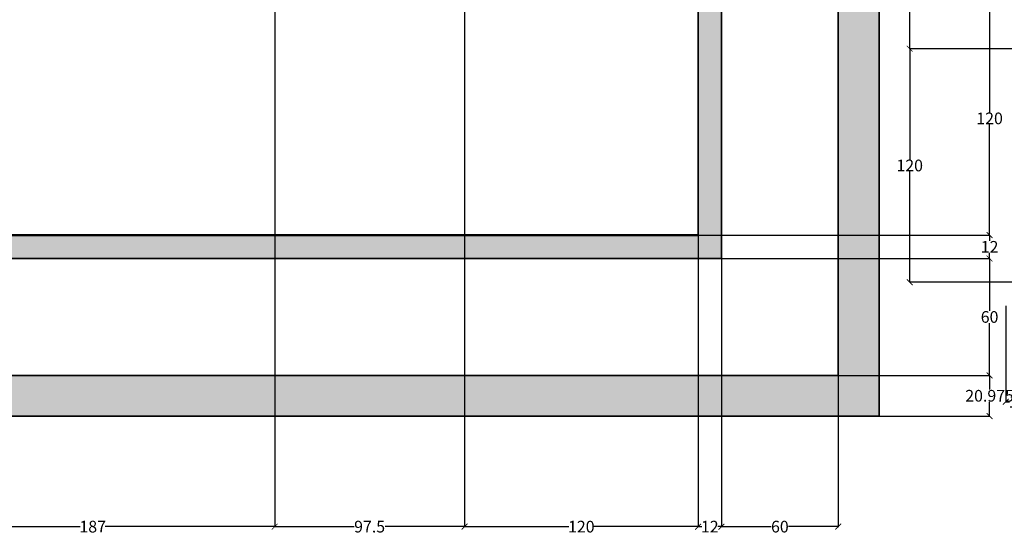
# Model space of a CAD drawing. Units: inches. Extents: x 925 to 2834, y 111 to 1355.
# Tile 5 of 25: x 1490 to 1996, y 111 to 376. Entities that reach past the tile are written whole.
import ezdxf

# ---------------------------------------------------------------- set-up
doc = ezdxf.new("R2010")
doc.units = ezdxf.units.IN
doc.header["$MEASUREMENT"] = 0
for name, color, linetype, lineweight in [('A-ANNO-DIMS', 2, 'Continuous', 18), ('A-ANNO-TTLB', 7, 'Continuous', 35), ('A-FLOR-PATT', 252, 'Continuous', 13), ('A-WALL', 7, 'Continuous', 50)]:
    doc.layers.add(name, color=color, linetype=linetype, lineweight=lineweight)
doc.styles.get("Standard").update_dxf_attribs({"font": 'arial.ttf'})
doc.dimstyles.get("Standard").update_dxf_attribs({"dimtxt": 6, "dimasz": 3, "dimexe": 0.18, "dimexo": 0.0625, "dimgap": 0.09, "dimtad": 0, "dimtih": 1, "dimtoh": 1, "dimdec": 1, "dimzin": 0, "dimdsep": 46, "dimlunit": 3, "dimtxsty": 'Standard', "dimblk": 'ARCHTICK', "dimcen": 0.09, "dimadec": 0, "dimazin": 0, "dimtfac": 1, "dimtdec": 1, "dimtofl": 0, "dimtmove": 0, "dimatfit": 3, "dimfxl": 1, "dimtolj": 1, "dimtzin": 0, "dimarcsym": 0})

# ---------------------------------------------------------------- blocks, each defined once
blk = doc.blocks.new('_ArchTick')
at = {"color": 0, "linetype": 'ByBlock', "const_width": 0.15}
blk.add_lwpolyline([(-0.5, -0.5), (0.5, 0.5)], dxfattribs=at)
blk = doc.blocks.new('*D27')
at = {"layer": 'A-ANNO-DIMS', "color": 0, "lineweight": -2, "transparency": 16777216}
for p, q in [((1621.21, 395.03), (1621.21, 115.18)), ((1434.21, 385.03), (1434.21, 115.18)), ((1434.21, 115.36), (1521.28, 115.36)), ((1621.21, 115.36), (1534.15, 115.36))]:
    blk.add_line(p, q, dxfattribs=at)
at = {"layer": 'Defpoints', "color": 0, "transparency": 16777216}
for p in [(1621.21, 395.09), (1434.21, 385.09), (1621.21, 115.36)]:
    blk.add_point(p, dxfattribs=at)
at = {"layer": 'A-ANNO-DIMS', "color": 0, "lineweight": -2, "transparency": 16777216, "xscale": 3, "yscale": 3, "zscale": 3, "rotation": 180}
blk.add_blockref('_ArchTick', (1434.21, 115.36), dxfattribs=at)
at = {"layer": 'A-ANNO-DIMS', "color": 0, "lineweight": -2, "transparency": 16777216, "xscale": 3, "yscale": 3, "zscale": 3}
blk.add_blockref('_ArchTick', (1621.21, 115.36), dxfattribs=at)
at = {"layer": 'A-ANNO-DIMS', "color": 0, "transparency": 16777216, "insert": (1527.71, 115.36), "char_height": 6, "attachment_point": 5}
blk.add_mtext('\\A1;187', dxfattribs=at)
blk = doc.blocks.new('*D28')
at = {"layer": 'A-ANNO-DIMS', "color": 0, "lineweight": -2, "transparency": 16777216}
for p, q in [((1621.21, 395.03), (1621.21, 115.18)), ((1718.71, 385.03), (1718.71, 115.18)), ((1621.21, 115.36), (1662.06, 115.36)), ((1718.71, 115.36), (1677.87, 115.36))]:
    blk.add_line(p, q, dxfattribs=at)
at = {"layer": 'Defpoints', "color": 0, "transparency": 16777216}
for p in [(1621.21, 395.09), (1718.71, 385.09), (1718.71, 115.36)]:
    blk.add_point(p, dxfattribs=at)
at = {"layer": 'A-ANNO-DIMS', "color": 0, "lineweight": -2, "transparency": 16777216, "xscale": 3, "yscale": 3, "zscale": 3, "rotation": 180}
blk.add_blockref('_ArchTick', (1621.21, 115.36), dxfattribs=at)
at = {"layer": 'A-ANNO-DIMS', "color": 0, "lineweight": -2, "transparency": 16777216, "xscale": 3, "yscale": 3, "zscale": 3}
blk.add_blockref('_ArchTick', (1718.71, 115.36), dxfattribs=at)
at = {"layer": 'A-ANNO-DIMS', "color": 0, "transparency": 16777216, "insert": (1669.96, 115.36), "char_height": 6, "attachment_point": 5}
blk.add_mtext('\\A1;97.5', dxfattribs=at)
blk = doc.blocks.new('*D29')
at = {"layer": 'A-ANNO-DIMS', "color": 0, "lineweight": -2, "transparency": 16777216}
for p, q in [((1718.71, 385.03), (1718.71, 115.18)), ((1838.71, 265.03), (1838.71, 115.18)), ((1718.71, 115.36), (1772.29, 115.36)), ((1838.71, 115.36), (1785.14, 115.36))]:
    blk.add_line(p, q, dxfattribs=at)
at = {"layer": 'Defpoints', "color": 0, "transparency": 16777216}
for p in [(1718.71, 385.09), (1838.71, 265.09), (1838.71, 115.36)]:
    blk.add_point(p, dxfattribs=at)
at = {"layer": 'A-ANNO-DIMS', "color": 0, "lineweight": -2, "transparency": 16777216, "xscale": 3, "yscale": 3, "zscale": 3, "rotation": 180}
blk.add_blockref('_ArchTick', (1718.71, 115.36), dxfattribs=at)
at = {"layer": 'A-ANNO-DIMS', "color": 0, "lineweight": -2, "transparency": 16777216, "xscale": 3, "yscale": 3, "zscale": 3}
blk.add_blockref('_ArchTick', (1838.71, 115.36), dxfattribs=at)
at = {"layer": 'A-ANNO-DIMS', "color": 0, "transparency": 16777216, "insert": (1778.71, 115.36), "char_height": 6, "attachment_point": 5}
blk.add_mtext('\\A1;120', dxfattribs=at)
blk = doc.blocks.new('*D30')
at = {"layer": 'A-ANNO-DIMS', "color": 0, "lineweight": -2, "transparency": 16777216}
for p, q in [((1838.71, 265.03), (1838.71, 115.18)), ((1850.71, 253.03), (1850.71, 115.18)), ((1838.71, 115.36), (1840.64, 115.36)), ((1850.71, 115.36), (1848.79, 115.36))]:
    blk.add_line(p, q, dxfattribs=at)
at = {"layer": 'Defpoints', "color": 0, "transparency": 16777216}
for p in [(1838.71, 265.09), (1850.71, 253.09), (1850.71, 115.36)]:
    blk.add_point(p, dxfattribs=at)
at = {"layer": 'A-ANNO-DIMS', "color": 0, "lineweight": -2, "transparency": 16777216, "xscale": 3, "yscale": 3, "zscale": 3, "rotation": 180}
blk.add_blockref('_ArchTick', (1838.71, 115.36), dxfattribs=at)
at = {"layer": 'A-ANNO-DIMS', "color": 0, "lineweight": -2, "transparency": 16777216, "xscale": 3, "yscale": 3, "zscale": 3}
blk.add_blockref('_ArchTick', (1850.71, 115.36), dxfattribs=at)
at = {"layer": 'A-ANNO-DIMS', "color": 0, "transparency": 16777216, "insert": (1844.71, 115.36), "char_height": 6, "attachment_point": 5}
blk.add_mtext('\\A1;12', dxfattribs=at)
blk = doc.blocks.new('*D31')
at = {"layer": 'A-ANNO-DIMS', "color": 0, "lineweight": -2, "transparency": 16777216}
for p, q in [((1850.71, 253.03), (1850.71, 115.18)), ((1910.71, 193.03), (1910.71, 115.18)), ((1850.71, 115.36), (1876.32, 115.36)), ((1910.71, 115.36), (1885.11, 115.36))]:
    blk.add_line(p, q, dxfattribs=at)
at = {"layer": 'Defpoints', "color": 0, "transparency": 16777216}
for p in [(1850.71, 253.09), (1910.71, 193.09), (1910.71, 115.36)]:
    blk.add_point(p, dxfattribs=at)
at = {"layer": 'A-ANNO-DIMS', "color": 0, "lineweight": -2, "transparency": 16777216, "xscale": 3, "yscale": 3, "zscale": 3, "rotation": 180}
blk.add_blockref('_ArchTick', (1850.71, 115.36), dxfattribs=at)
at = {"layer": 'A-ANNO-DIMS', "color": 0, "lineweight": -2, "transparency": 16777216, "xscale": 3, "yscale": 3, "zscale": 3}
blk.add_blockref('_ArchTick', (1910.71, 115.36), dxfattribs=at)
at = {"layer": 'A-ANNO-DIMS', "color": 0, "transparency": 16777216, "insert": (1880.71, 115.36), "char_height": 6, "attachment_point": 5}
blk.add_mtext('\\A1;60', dxfattribs=at)
blk = doc.blocks.new('*D40')
at = {"layer": 'A-ANNO-DIMS', "color": 0, "lineweight": -2, "transparency": 16777216}
for p, q in [((1910.78, 193.09), (1988.62, 193.09)), ((1988.44, 193.09), (1988.44, 185.75)), ((1988.44, 172.11), (1988.44, 179.45)), ((1931.75, 172.11), (1988.62, 172.11))]:
    blk.add_line(p, q, dxfattribs=at)
at = {"layer": 'Defpoints', "color": 0, "transparency": 16777216}
for p in [(1910.71, 193.09), (1988.44, 193.09), (1931.69, 172.11)]:
    blk.add_point(p, dxfattribs=at)
at = {"layer": 'A-ANNO-DIMS', "color": 0, "lineweight": -2, "transparency": 16777216, "xscale": 3, "yscale": 3, "zscale": 3}
for p, rotation in [((1988.44, 193.09), 90), ((1988.44, 172.11), 270)]:
    blk.add_blockref('_ArchTick', p, dxfattribs=dict(at, rotation=rotation))
at = {"layer": 'A-ANNO-DIMS', "color": 0, "transparency": 16777216, "insert": (1988.44, 182.6), "char_height": 6, "attachment_point": 5}
blk.add_mtext('\\A1;20.975', dxfattribs=at)
blk = doc.blocks.new('*D41')
at = {"layer": 'A-ANNO-DIMS', "color": 0, "lineweight": -2, "transparency": 16777216}
for p, q in [((1850.78, 253.09), (1988.62, 253.09)), ((1988.44, 253.09), (1988.44, 226.24)), ((1988.44, 193.09), (1988.44, 219.94)), ((1910.78, 193.09), (1988.62, 193.09))]:
    blk.add_line(p, q, dxfattribs=at)
at = {"layer": 'Defpoints', "color": 0, "transparency": 16777216}
for p in [(1850.71, 253.09), (1988.44, 253.09), (1910.71, 193.09)]:
    blk.add_point(p, dxfattribs=at)
at = {"layer": 'A-ANNO-DIMS', "color": 0, "lineweight": -2, "transparency": 16777216, "xscale": 3, "yscale": 3, "zscale": 3}
for p, rotation in [((1988.44, 253.09), 90), ((1988.44, 193.09), 270)]:
    blk.add_blockref('_ArchTick', p, dxfattribs=dict(at, rotation=rotation))
at = {"layer": 'A-ANNO-DIMS', "color": 0, "transparency": 16777216, "insert": (1988.44, 223.09), "char_height": 6, "attachment_point": 5}
blk.add_mtext('\\A1;60', dxfattribs=at)
blk = doc.blocks.new('*D42')
at = {"layer": 'A-ANNO-DIMS', "color": 0, "lineweight": -2, "transparency": 16777216}
for p, q in [((1838.78, 265.09), (1988.62, 265.09)), ((1988.44, 265.09), (1988.44, 262.19)), ((1850.78, 253.09), (1988.62, 253.09)), ((1988.44, 253.09), (1988.44, 255.99))]:
    blk.add_line(p, q, dxfattribs=at)
at = {"layer": 'Defpoints', "color": 0, "transparency": 16777216}
for p in [(1838.71, 265.09), (1988.44, 265.09), (1850.71, 253.09)]:
    blk.add_point(p, dxfattribs=at)
at = {"layer": 'A-ANNO-DIMS', "color": 0, "lineweight": -2, "transparency": 16777216, "xscale": 3, "yscale": 3, "zscale": 3}
for p, rotation in [((1988.44, 265.09), 90), ((1988.44, 253.09), 270)]:
    blk.add_blockref('_ArchTick', p, dxfattribs=dict(at, rotation=rotation))
at = {"layer": 'A-ANNO-DIMS', "color": 0, "transparency": 16777216, "insert": (1988.44, 259.09), "char_height": 6, "attachment_point": 5}
blk.add_mtext('\\A1;12', dxfattribs=at)
blk = doc.blocks.new('*D43')
at = {"layer": 'A-ANNO-DIMS', "color": 0, "lineweight": -2, "transparency": 16777216}
for p, q in [((1718.78, 385.09), (1988.62, 385.09)), ((1988.44, 385.09), (1988.44, 328.24)), ((1988.44, 265.09), (1988.44, 321.94)), ((1838.78, 265.09), (1988.62, 265.09))]:
    blk.add_line(p, q, dxfattribs=at)
at = {"layer": 'Defpoints', "color": 0, "transparency": 16777216}
for p in [(1718.71, 385.09), (1988.44, 385.09), (1838.71, 265.09)]:
    blk.add_point(p, dxfattribs=at)
at = {"layer": 'A-ANNO-DIMS', "color": 0, "lineweight": -2, "transparency": 16777216, "xscale": 3, "yscale": 3, "zscale": 3}
for p, rotation in [((1988.44, 385.09), 90), ((1988.44, 265.09), 270)]:
    blk.add_blockref('_ArchTick', p, dxfattribs=dict(at, rotation=rotation))
at = {"layer": 'A-ANNO-DIMS', "color": 0, "transparency": 16777216, "insert": (1988.44, 325.09), "char_height": 6, "attachment_point": 5}
blk.add_mtext('\\A1;120', dxfattribs=at)
blk = doc.blocks.new('*D62')
at = {"layer": 'A-ANNO-DIMS', "color": 0, "lineweight": -2, "transparency": 16777216}
for p, q in [((2008.76, 240.83), (2008.76, 179.37)), ((1996.76, 228.83), (1996.76, 179.37)), ((1996.76, 179.55), (1998.68, 179.55)), ((2008.76, 179.55), (2006.83, 179.55))]:
    blk.add_line(p, q, dxfattribs=at)
at = {"layer": 'Defpoints', "color": 0, "transparency": 16777216}
for p in [(2008.76, 240.9), (1996.76, 228.9), (2008.76, 179.55)]:
    blk.add_point(p, dxfattribs=at)
at = {"layer": 'A-ANNO-DIMS', "color": 0, "lineweight": -2, "transparency": 16777216, "xscale": 3, "yscale": 3, "zscale": 3, "rotation": 180}
blk.add_blockref('_ArchTick', (1996.76, 179.55), dxfattribs=at)
at = {"layer": 'A-ANNO-DIMS', "color": 0, "lineweight": -2, "transparency": 16777216, "xscale": 3, "yscale": 3, "zscale": 3}
blk.add_blockref('_ArchTick', (2008.76, 179.55), dxfattribs=at)
at = {"layer": 'A-ANNO-DIMS', "color": 0, "transparency": 16777216, "insert": (2002.76, 179.55), "char_height": 6, "attachment_point": 5}
blk.add_mtext('\\A1;12', dxfattribs=at)
blk = doc.blocks.new('*D75')
at = {"layer": 'A-ANNO-DIMS', "color": 0, "lineweight": -2, "transparency": 16777216}
for p, q in [((2124.2, 360.9), (1947.23, 360.9)), ((1947.41, 360.9), (1947.41, 304.05)), ((1947.41, 240.9), (1947.41, 297.74)), ((2008.7, 240.9), (1947.23, 240.9))]:
    blk.add_line(p, q, dxfattribs=at)
at = {"layer": 'Defpoints', "color": 0, "transparency": 16777216}
for p in [(1947.41, 360.9), (2124.26, 360.9), (2008.76, 240.9)]:
    blk.add_point(p, dxfattribs=at)
at = {"layer": 'A-ANNO-DIMS', "color": 0, "lineweight": -2, "transparency": 16777216, "xscale": 3, "yscale": 3, "zscale": 3}
for p, rotation in [((1947.41, 360.9), 90), ((1947.41, 240.9), 270)]:
    blk.add_blockref('_ArchTick', p, dxfattribs=dict(at, rotation=rotation))
at = {"layer": 'A-ANNO-DIMS', "color": 0, "transparency": 16777216, "insert": (1947.41, 300.9), "char_height": 6, "attachment_point": 5}
blk.add_mtext('\\A1;120', dxfattribs=at)
blk = doc.blocks.new('*D76')
at = {"layer": 'A-ANNO-DIMS', "color": 0, "lineweight": -2, "transparency": 16777216}
for p, q in [((2124.2, 500.4), (1947.23, 500.4)), ((1947.41, 500.4), (1947.41, 433.8)), ((1947.41, 360.9), (1947.41, 427.49)), ((2124.2, 360.9), (1947.23, 360.9))]:
    blk.add_line(p, q, dxfattribs=at)
at = {"layer": 'Defpoints', "color": 0, "transparency": 16777216}
for p in [(1947.41, 500.4), (2124.26, 500.4), (2124.26, 360.9)]:
    blk.add_point(p, dxfattribs=at)
at = {"layer": 'A-ANNO-DIMS', "color": 0, "lineweight": -2, "transparency": 16777216, "xscale": 3, "yscale": 3, "zscale": 3}
for p, rotation in [((1947.41, 500.4), 90), ((1947.41, 360.9), 270)]:
    blk.add_blockref('_ArchTick', p, dxfattribs=dict(at, rotation=rotation))
at = {"layer": 'A-ANNO-DIMS', "color": 0, "transparency": 16777216, "insert": (1947.41, 430.65), "char_height": 6, "attachment_point": 5}
blk.add_mtext('\\A1;139.5', dxfattribs=at)

msp = doc.modelspace()

# ---------------------------------------------------------------- hatches: boundary and pattern name
at = {"layer": 'A-FLOR-PATT', "transparency": 33554605}
h = msp.add_hatch(color=256, dxfattribs=at)
h.dxf.hatch_style = 1
h.paths.add_polyline_path([(1931.688, 1294.5638), (991.7375, 1294.5638), (991.7375, 172.1134), (1931.688, 172.1134)])
h.paths.add_polyline_path([(1910.7128, 1273.5886), (1910.7128, 193.0886), (1012.7128, 193.0886), (1012.7128, 1273.5886)], flags=16)
h.paths.add_polyline_path([(1850.7128, 1213.5886), (1850.7128, 253.0886), (1072.7128, 253.0886), (1072.7128, 1213.5886)], flags=0)
h.paths.add_polyline_path([(1838.7128, 1201.5886), (1838.7128, 265.0886), (1084.7128, 265.0886), (1084.7128, 530.5886), (1084.7128, 1201.5886)], flags=0)
h.paths.add_polyline_path([(1547.6758, 1155.7396), (1547.6758, 1119.115), (1513.0687, 1119.115), (1513.0687, 1155.7396)], flags=0)
h.paths.add_polyline_path([(1600.1067, 1154.9439), (1634.7139, 1154.9439), (1634.7139, 1119.115), (1600.1067, 1119.115)], flags=0)
h.paths.add_polyline_path([(1505.2502, 1144.5358), (1505.2502, 1119.115), (1470.643, 1119.115), (1470.643, 1144.5358)], flags=0)
h.paths.add_polyline_path([(1559.1357, 1141.0962), (1593.7428, 1141.0962), (1593.7428, 1119.115), (1559.1357, 1119.115)], flags=0)
h.paths.add_polyline_path([(1462.8966, 1154.9439), (1462.8966, 1119.115), (1428.2895, 1119.115), (1428.2895, 1154.9439)], flags=0)
h.paths.add_polyline_path([(1642.4603, 1144.5358), (1677.0675, 1144.5358), (1677.0675, 1119.115), (1642.4603, 1119.115)], flags=0)
h.paths.add_polyline_path([(1422.3508, 1141.0962), (1422.3508, 1119.115), (1387.7436, 1119.115), (1387.7436, 1141.0962)], flags=0)
h.paths.add_polyline_path([(1684.8859, 1155.7396), (1719.4931, 1155.7396), (1719.4931, 1119.115), (1684.8859, 1119.115)], flags=0)
h.paths.add_polyline_path([(1718.7128, 1081.5886), (1718.7128, 1050.1249), (1715.7128, 1050.1249), (1715.7128, 1026.1249), (1715.7128, 1002.1249), (1718.7128, 1002.1249), (1730.7128, 1002.1249), (1730.7128, 998.1249), (1730.7128, 990.1249), (1730.7128, 986.1249), (1718.7128, 986.1249), (1718.7128, 893.5886), (1715.3735, 893.5886), (1715.3735, 891.5886), (1713.3735, 891.5886, 0.41421356), (1677.3735, 855.5886), (1713.3735, 855.5886), (1713.3735, 853.5886), (1715.3735, 853.5886), (1715.3735, 851.5886), (1718.7128, 851.5886), (1718.7128, 821.5865), (1734.4655, 821.5865), (1734.3735, 819.5886, -0.41421356), (1712.4415, 793.5886), (1712.4415, 791.5886), (1718.7128, 791.5886), (1718.7128, 717.5886), (1718.7128, 669.5886), (1732.7128, 669.5886), (1732.7128, 665.5886), (1732.7128, 641.5886), (1732.7128, 634.5886), (1732.7128, 610.5886), (1732.7128, 603.5886), (1718.7128, 603.5886), (1718.7128, 385.0886), (1434.2128, 385.0886), (1434.2128, 530.5886), (1410.2128, 530.5886), (1408.2128, 530.5886), (1408.2128, 532.5886, 0.41421356), (1372.2128, 568.5886), (1372.2128, 532.5886), (1370.2128, 532.5886), (1370.2128, 530.5886), (1368.2128, 530.5886), (1282.2128, 530.5886), (1210.2128, 530.5886), (1200.2128, 530.5886), (1200.2128, 542.1915), (1183.2307, 542.1915), (1183.2307, 546.1915), (1200.2128, 546.1915), (1200.2128, 572.1915), (1183.2307, 572.1915), (1183.2307, 576.1915), (1200.2128, 576.1915), (1200.2128, 727.5886), (1210.2128, 727.5886), (1234.2128, 727.5886), (1259.7128, 727.5886), (1259.7128, 775.5886), (1259.7128, 799.5886), (1259.7128, 847.5886), (1259.7128, 993.5872), (1259.7128, 1065.5872), (1259.7128, 1071.5886), (1219.6318, 1071.5886), (1219.6318, 1081.5886), (1084.7128, 1081.5886), (1084.7128, 1119.115), (1256.8974, 1119.115), (1256.8974, 1154.9439), (1291.5046, 1154.9439), (1291.5046, 1119.115), (1256.8974, 1119.115), (1256.6723, 1081.5886), (1293.7128, 1081.5886), (1341.7128, 1081.5886), (1341.7128, 1093.5886), (1347.7128, 1093.5886), (1371.7128, 1093.5886), (1377.7128, 1093.5886), (1377.7128, 1081.5886), (1668.7128, 1081.5886), (1668.7128, 1117.5886), (1675.7128, 1117.5886), (1711.7128, 1117.5886), (1718.7128, 1117.5886)], flags=0)
h.paths.add_polyline_path([(1376.2838, 1155.7396), (1376.2838, 1119.115), (1341.6766, 1119.115), (1341.6766, 1155.7396)], flags=0)
h.paths.add_polyline_path([(1341.7128, 1076.0886), (1293.7128, 1076.0886), (1293.7128, 1071.5886), (1269.7128, 1071.5886), (1269.7128, 1065.5872), (1266.7128, 1065.5872), (1266.7128, 1029.5872), (1265.7128, 1029.5872), (1265.7128, 993.5872), (1269.7128, 993.5872), (1269.7128, 903.5886), (1269.7128, 893.5886), (1269.7128, 847.5886), (1265.2128, 847.5886), (1265.2128, 799.5886), (1269.7128, 799.5886), (1269.7128, 775.5886), (1265.2128, 775.5886), (1265.2128, 727.5886), (1269.7128, 727.5886), (1444.2128, 727.5886), (1444.2128, 717.5886), (1234.2128, 717.5886), (1234.2128, 722.0886), (1210.2128, 722.0886), (1210.2128, 717.5886), (1210.2128, 540.5886), (1210.2128, 536.0886), (1282.2128, 536.0886), (1282.2128, 535.0886), (1210.2128, 535.0886), (1210.2128, 540.5886), (1210.2128, 717.5886), (1210.2128, 723.0886), (1234.2128, 723.0886), (1234.2128, 717.5886), (1444.2128, 717.5886), (1444.2128, 727.5886), (1269.7128, 727.5886), (1264.2128, 727.5886), (1264.2128, 775.5886), (1269.7128, 775.5886), (1269.7128, 799.5886), (1264.2128, 799.5886), (1264.2128, 847.5886), (1269.7128, 847.5886), (1269.7128, 893.5886), (1269.7128, 903.5886), (1269.7128, 993.5872), (1264.7128, 993.5872), (1264.7128, 1029.5872), (1265.7128, 1029.5872), (1265.7128, 1065.5872), (1269.7128, 1065.5872), (1269.7128, 1071.5886), (1293.7128, 1071.5886), (1293.7128, 1077.0886), (1341.7128, 1077.0886)], flags=0)
h.paths.add_polyline_path([(1730.9529, 1141.0962), (1765.5601, 1141.0962), (1765.5601, 1119.115), (1730.9529, 1119.115)], flags=0)
h.paths.add_polyline_path([(1333.8582, 1144.5358), (1333.8582, 1119.115), (1299.251, 1119.115), (1299.251, 1144.5358)], flags=0)
h.paths.add_polyline_path([(1592.7128, 968.5886), (1596.0342, 968.5886), (1602.7128, 968.5886), (1708.7128, 968.5886), (1708.7128, 903.5886), (1602.7128, 903.5886), (1602.7128, 938.5886), (1592.7128, 938.5886), (1592.7128, 903.5886), (1451.7128, 903.5886), (1451.7128, 893.5886), (1511.7128, 893.5886), (1511.7128, 881.5886), (1515.2128, 881.5886), (1518.7128, 881.5886), (1518.7128, 893.5886), (1592.7128, 893.5886), (1592.7128, 799.5886), (1518.7128, 799.5886), (1518.7128, 857.5886), (1511.7128, 857.5886), (1511.7128, 799.5886), (1511.7128, 772.0886), (1521.7128, 772.0886), (1521.7128, 792.5886), (1592.7128, 792.5886), (1592.7128, 727.5886), (1521.7128, 727.5886), (1521.7128, 748.0886), (1511.7128, 748.0886), (1511.7128, 717.5886), (1708.7128, 717.5886), (1714.2128, 717.5886), (1714.2128, 669.5886), (1708.7128, 669.5886), (1708.7128, 641.5886), (1492.2128, 641.5886), (1492.2128, 631.5886), (1621.2128, 631.5886), (1621.2128, 443.0886), (1625.7128, 443.0886), (1625.7128, 503.0886), (1625.7128, 507.5886), (1625.7128, 631.5886), (1708.7128, 631.5886), (1708.7128, 507.5886), (1655.7128, 507.5886), (1655.7128, 503.0886), (1708.7128, 503.0886), (1708.7128, 395.0886), (1625.7128, 395.0886), (1625.7128, 419.0886), (1621.2128, 419.0886), (1621.2128, 395.0886), (1482.2128, 395.0886), (1482.2128, 385.0886), (1434.2128, 385.0886), (1434.2128, 433.0886), (1444.2128, 433.0886), (1444.2128, 631.5886), (1450.2128, 631.5886), (1450.2128, 634.91), (1452.2128, 634.91), (1452.2128, 669.5886), (1454.2128, 669.5886, -0.40021217), (1490.1712, 635.3173), (1492.2128, 635.3173), (1492.2128, 641.5886), (1564.7128, 641.5886), (1564.7128, 677.5886), (1672.7128, 677.5886), (1672.7128, 681.5886), (1564.7128, 681.5886), (1564.7128, 717.5886), (1511.7128, 717.5886), (1511.7128, 748.0886), (1511.7128, 772.0886), (1511.7128, 799.5886), (1511.7128, 857.5886), (1511.8913, 857.5886), (1511.8913, 859.5886), (1515.6201, 859.5886, 0.41421356), (1537.552, 879.5886), (1513.552, 879.5886), (1511.8913, 879.5886), (1511.8913, 881.5886), (1511.7128, 881.5886), (1511.7128, 893.5886), (1451.7128, 893.5886), (1451.7128, 903.5886), (1592.7128, 903.5886), (1592.7128, 938.5886), (1592.7128, 940.5886), (1596.4415, 940.5886, 0.41421356), (1618.3735, 966.5886), (1594.3735, 966.5886), (1592.7128, 966.5886)], flags=0)
h.paths.add_polyline_path([(1377.7128, 903.5886), (1377.7128, 893.5886), (1305.7128, 893.5886), (1305.7128, 903.5886)], flags=0)
h.paths.add_polyline_path([(1708.7128, 821.5886), (1712.0342, 821.5886), (1712.0342, 819.5886), (1710.3735, 819.5886), (1708.7128, 819.5886)], flags=0)
h.paths.add_polyline_path([(1576.7128, 695.1992), (1575.5896, 693.6649), (1575.9687, 694.6994), (1575.4438, 695.1992), (1575.9687, 695.699), (1575.5896, 696.7335)], flags=0)
h.paths.add_polyline_path([(1565.9817, 662.3134), (1565.4568, 661.8136), (1565.8359, 660.7791), (1564.7128, 662.3134), (1565.8359, 663.8477), (1565.4568, 662.8132)], flags=0)
h.paths.add_polyline_path([(1444.2128, 433.0886), (1444.2128, 395.0886), (1482.2128, 395.0886), (1482.2128, 389.0886), (1438.2128, 389.0886), (1438.2128, 391.8608), (1438.2128, 433.0886)], flags=0)
h.paths.add_polyline_path([(1410.2128, 506.5886), (1410.2128, 289.0886), (1108.7128, 289.0886), (1108.7128, 506.5886)], flags=0)
h.paths.add_polyline_path([(1612.3153, 838.3016), (1680.4151, 838.3016), (1680.4151, 851.3131), (1612.3153, 851.3131)], flags=8)
h.paths.add_polyline_path([(1208.3174, 395.0436), (1282.1017, 395.0436), (1282.1017, 408.0552), (1208.3174, 408.0552)], flags=8)
h.paths.add_polyline_path([(1291.8049, 598.7427), (1369.8017, 598.7427), (1369.8017, 611.7542), (1291.8049, 611.7542)], flags=8)
h.paths.add_polyline_path([(1119.679, 917.3022), (1191.0817, 917.3022), (1191.0817, 930.3137), (1119.679, 930.3137)], flags=8)
h.paths.add_polyline_path([(1332.2261, 815.9808), (1410.2258, 815.9808), (1410.2258, 829.001), (1332.2261, 829.001)], flags=8)
h.paths.add_polyline_path([(1390.9013, 955.8158), (1475.4981, 955.8158), (1475.4981, 968.8273), (1390.9013, 968.8273)], flags=8)
h.paths.add_polyline_path([(1620.3436, 998.9325), (1688.4434, 998.9325), (1688.4434, 1011.944), (1620.3436, 1011.944)], flags=8)
h.paths.add_polyline_path([(1620.3436, 914.1039), (1691.7405, 914.1039), (1691.7405, 927.1155), (1620.3436, 927.1155)], flags=8)
h.paths.add_polyline_path([(1521.4542, 816.005), (1589.5569, 816.005), (1589.5569, 829.0253), (1521.4542, 829.0253)], flags=8)
h.paths.add_polyline_path([(1528.524, 740.3497), (1602.3082, 740.3497), (1602.3082, 753.3613), (1528.524, 753.3613)], flags=8)
h.paths.add_polyline_path([(1627.6094, 762.6128), (1702.3091, 762.6128), (1702.3091, 775.6244), (1627.6094, 775.6244)], flags=8)
h.paths.add_polyline_path([(1610.5442, 657.2751), (1684.3284, 657.2751), (1684.3284, 670.2867), (1610.5442, 670.2867)], flags=8)
h.paths.add_polyline_path([(1636.6983, 519.472), (1711.3981, 519.472), (1711.3981, 532.4835), (1636.6983, 532.4835)], flags=8)
h.paths.add_polyline_path([(1616.8577, 424.8539), (1694.8545, 424.8539), (1694.8545, 437.8654), (1616.8577, 437.8654)], flags=8)
h.paths.add_polyline_path([(1506.1456, 460.8838), (1579.9299, 460.8838), (1579.9299, 473.8953), (1506.1456, 473.8953)], flags=8)
h.paths.add_polyline_path([(1624.6119, 784.6011), (1696.9185, 784.6011), (1696.9185, 797.7864), (1624.6119, 797.7864)], flags=8)
h.paths.add_polyline_path([(1606.3732, 854.2194), (1683.3039, 854.2194), (1683.3039, 867.4048), (1606.3732, 867.4048)], flags=8)
h.paths.add_polyline_path([(1127.8008, 940.3581), (1165.1637, 940.3581), (1165.1637, 953.5348), (1127.8008, 953.5348)], flags=8)
h.paths.add_polyline_path([(1620.8657, 1019.4968), (1677.3447, 1019.4968), (1677.3447, 1032.6735), (1620.8657, 1032.6735)], flags=8)
h.paths.add_polyline_path([(1620.8643, 930.1821), (1703.0564, 930.1821), (1703.0564, 943.3675), (1620.8643, 943.3675)], flags=8)
h.paths.add_polyline_path([(1324.5702, 836.8338), (1408.0892, 836.8338), (1408.0892, 850.0191), (1324.5702, 850.0191)], flags=8)
h.paths.add_polyline_path([(1281.6584, 622.8885), (1383.6213, 622.8885), (1383.6213, 636.0739), (1281.6584, 636.0739)], flags=8)
h.paths.add_polyline_path([(1210.6721, 416.7893), (1269.1299, 416.7893), (1269.1299, 429.9747), (1210.6721, 429.9747)], flags=8)
h.paths.add_polyline_path([(1507.8264, 477.4836), (1586.7329, 477.4836), (1586.7329, 490.669), (1507.8264, 490.669)], flags=8)
h.paths.add_polyline_path([(1643.6238, 443.8135), (1696.6696, 443.8135), (1696.6696, 456.5643), (1643.6238, 456.5643)], flags=8)
h.paths.add_polyline_path([(1647.2466, 540.5638), (1693.1825, 540.5638), (1693.1825, 553.7491), (1647.2466, 553.7491)], flags=8)
h.paths.add_polyline_path([(1626.0633, 668.5064), (1673.3174, 668.5064), (1673.3174, 681.6831), (1626.0633, 681.6831)], flags=8)
h.paths.add_polyline_path([(1538.2915, 830.7872), (1567.5942, 830.7872), (1567.5942, 843.5293), (1538.2915, 843.5293)], flags=8)
h.paths.add_polyline_path([(1530.9338, 754.0477), (1559.576, 754.0477), (1559.576, 766.7898), (1530.9338, 766.7898)], flags=8)
h.paths.add_polyline_path([(1351.2461, 979.2309), (1513.8919, 979.2309), (1513.8919, 992.4076), (1351.2461, 992.4076)], flags=8)
at = {"layer": 'A-FLOR-PATT'}
h = msp.add_hatch(color=256, dxfattribs=at)
h.dxf.hatch_style = 1
h.paths.add_polyline_path([(1850.7128, 1213.5886), (1072.7128, 1213.5886), (1072.7128, 253.0886), (1850.7128, 253.0886)])
h.paths.add_polyline_path([(1084.7128, 1201.5886), (1838.7128, 1201.5886), (1838.7128, 265.0886), (1084.7128, 265.0886)], flags=16)
h.paths.add_polyline_path([(1183.2307, 576.1915), (1200.2128, 576.1915), (1200.2128, 727.5886), (1210.2128, 727.5886), (1234.2128, 727.5886), (1259.7128, 727.5886), (1259.7128, 775.5886), (1259.7128, 799.5886), (1259.7128, 847.5886), (1259.7128, 993.5872), (1259.7128, 1065.5872), (1259.7128, 1071.5886), (1219.6318, 1071.5886), (1219.6318, 1081.5886), (1293.7128, 1081.5886), (1341.7128, 1081.5886), (1341.7128, 1093.5886), (1347.7128, 1093.5886), (1347.7128, 1081.5886), (1371.7128, 1081.5886), (1371.7128, 1093.5886), (1377.7128, 1093.5886), (1377.7128, 1081.5886), (1668.7128, 1081.5886), (1668.7128, 1117.5886), (1675.7128, 1117.5886), (1675.7128, 1081.5886), (1711.7128, 1081.5886), (1711.7128, 1117.5886), (1718.7128, 1117.5886), (1718.7128, 1081.5886), (1718.7128, 1050.1249), (1715.7128, 1050.1249), (1715.7128, 1026.1249), (1715.7128, 1002.1249), (1718.7128, 1002.1249), (1730.7128, 1002.1249), (1730.7128, 998.1249), (1730.7128, 990.1249), (1730.7128, 986.1249), (1718.7128, 986.1249), (1718.7128, 893.5886), (1715.3735, 893.5886), (1715.3735, 891.5886), (1713.3735, 891.5886, 0.41421356), (1677.3735, 855.5886), (1713.3735, 855.5886), (1713.3735, 853.5886), (1715.3735, 853.5886), (1715.3735, 851.5886), (1718.7128, 851.5886), (1718.7128, 821.5865), (1734.4655, 821.5865), (1734.3735, 819.5886, -0.41421356), (1712.4415, 793.5886), (1712.4415, 791.5886), (1718.7128, 791.5886), (1718.7128, 717.5886), (1718.7128, 669.5886), (1732.7128, 669.5886), (1732.7128, 665.5886), (1732.7128, 641.5886), (1732.7128, 634.5886), (1732.7128, 610.5886), (1732.7128, 603.5886), (1718.7128, 603.5886), (1718.7128, 385.0886), (1434.2128, 385.0886), (1434.2128, 433.0886), (1434.2128, 530.5886), (1410.2128, 530.5886), (1408.2128, 530.5886), (1408.2128, 532.5886, 0.41421356), (1372.2128, 568.5886), (1372.2128, 532.5886), (1370.2128, 532.5886), (1370.2128, 530.5886), (1368.2128, 530.5886), (1282.2128, 530.5886), (1210.2128, 530.5886), (1200.2128, 530.5886), (1200.2128, 542.1915), (1183.2307, 542.1915), (1183.2307, 546.1915), (1200.2128, 546.1915), (1200.2128, 572.1915), (1183.2307, 572.1915)], flags=0)
h.paths.add_polyline_path([(1210.2128, 717.5886), (1210.2128, 723.0886), (1234.2128, 723.0886), (1234.2128, 717.5886), (1444.2128, 717.5886), (1444.2128, 727.5886), (1269.7128, 727.5886), (1264.2128, 727.5886), (1264.2128, 775.5886), (1269.7128, 775.5886), (1269.7128, 799.5886), (1264.2128, 799.5886), (1264.2128, 847.5886), (1269.7128, 847.5886), (1269.7128, 893.5886), (1269.7128, 903.5886), (1269.7128, 993.5872), (1264.7128, 993.5872), (1264.7128, 1029.5872), (1265.7128, 1029.5872), (1265.7128, 1065.5872), (1269.7128, 1065.5872), (1269.7128, 1071.5886), (1293.7128, 1071.5886), (1293.7128, 1077.0886), (1341.7128, 1077.0886), (1341.7128, 1076.0886), (1293.7128, 1076.0886), (1293.7128, 1071.5886), (1269.7128, 1071.5886), (1269.7128, 1065.5872), (1266.7128, 1065.5872), (1266.7128, 1029.5872), (1265.7128, 1029.5872), (1265.7128, 993.5872), (1269.7128, 993.5872), (1269.7128, 903.5886), (1269.7128, 893.5886), (1269.7128, 847.5886), (1265.2128, 847.5886), (1265.2128, 799.5886), (1269.7128, 799.5886), (1269.7128, 775.5886), (1265.2128, 775.5886), (1265.2128, 727.5886), (1269.7128, 727.5886), (1444.2128, 727.5886), (1444.2128, 717.5886), (1234.2128, 717.5886), (1234.2128, 722.0886), (1210.2128, 722.0886), (1210.2128, 717.5886), (1210.2128, 540.5886), (1210.2128, 536.0886), (1282.2128, 536.0886), (1282.2128, 535.0886), (1210.2128, 535.0886), (1210.2128, 540.5886)], flags=0)
h.paths.add_polyline_path([(1450.2128, 634.91), (1452.2128, 634.91), (1452.2128, 669.5886), (1454.2128, 669.5886, -0.40021217), (1490.1712, 635.3173), (1492.2128, 635.3173), (1492.2128, 641.5886), (1564.7128, 641.5886), (1564.7128, 677.5886), (1672.7128, 677.5886), (1672.7128, 681.5886), (1564.7128, 681.5886), (1564.7128, 717.5886), (1511.7128, 717.5886), (1511.7128, 748.0886), (1511.7128, 772.0886), (1511.7128, 799.5886), (1511.7128, 857.5886), (1511.8913, 857.5886), (1511.8913, 859.5886), (1515.6201, 859.5886, 0.41421356), (1537.552, 879.5886), (1513.552, 879.5886), (1511.8913, 879.5886), (1511.8913, 881.5886), (1511.7128, 881.5886), (1511.7128, 893.5886), (1451.7128, 893.5886), (1451.7128, 903.5886), (1592.7128, 903.5886), (1592.7128, 938.5886), (1592.7128, 940.5886), (1596.4415, 940.5886, 0.41421356), (1618.3735, 966.5886), (1594.3735, 966.5886), (1592.7128, 966.5886), (1592.7128, 968.5886), (1596.0342, 968.5886), (1602.7128, 968.5886), (1708.7128, 968.5886), (1708.7128, 903.5886), (1602.7128, 903.5886), (1602.7128, 938.5886), (1592.7128, 938.5886), (1592.7128, 903.5886), (1451.7128, 903.5886), (1451.7128, 893.5886), (1511.7128, 893.5886), (1511.7128, 881.5886), (1518.7128, 881.5886), (1518.7128, 893.5886), (1592.7128, 893.5886), (1592.7128, 799.5886), (1518.7128, 799.5886), (1518.7128, 857.5886), (1511.7128, 857.5886), (1511.7128, 799.5886), (1511.7128, 772.0886), (1521.7128, 772.0886), (1521.7128, 792.5886), (1592.7128, 792.5886), (1592.7128, 727.5886), (1521.7128, 727.5886), (1521.7128, 748.0886), (1511.7128, 748.0886), (1511.7128, 717.5886), (1708.7128, 717.5886), (1714.2128, 717.5886), (1714.2128, 669.5886), (1708.7128, 669.5886), (1708.7128, 641.5886), (1492.2128, 641.5886), (1492.2128, 631.5886), (1621.2128, 631.5886), (1621.2128, 443.0886), (1625.7128, 443.0886), (1625.7128, 503.0886), (1625.7128, 507.5886), (1625.7128, 631.5886), (1708.7128, 631.5886), (1708.7128, 507.5886), (1655.7128, 507.5886), (1655.7128, 503.0886), (1708.7128, 503.0886), (1708.7128, 395.0886), (1625.7128, 395.0886), (1625.7128, 419.0886), (1621.2128, 419.0886), (1621.2128, 395.0886), (1482.2128, 395.0886), (1482.2128, 389.0886), (1438.2128, 389.0886), (1438.2128, 391.8608), (1438.2128, 433.0886), (1444.2128, 433.0886), (1444.2128, 631.5886), (1450.2128, 631.5886)], flags=0)
h.paths.add_polyline_path([(1444.2128, 433.0886), (1444.2128, 395.0886), (1482.2128, 395.0886), (1482.2128, 391.0886), (1440.2128, 391.0886), (1440.2128, 391.8608), (1440.2128, 433.0886)], flags=0)
h.paths.add_polyline_path([(1305.7128, 893.5886), (1305.7128, 903.5886), (1377.7128, 903.5886), (1377.7128, 893.5886)], flags=0)
h.paths.add_polyline_path([(1564.7128, 662.3134), (1565.8359, 663.8477), (1565.4568, 662.8132), (1565.9817, 662.3134), (1565.4568, 661.8136), (1565.8359, 660.7791)], flags=0)
h.paths.add_polyline_path([(1575.4438, 695.1992), (1575.9687, 695.699), (1575.5896, 696.7335), (1576.7128, 695.1992), (1575.5896, 693.6649), (1575.9687, 694.6994)], flags=0)
h.paths.add_polyline_path([(1708.7128, 821.5886), (1712.0342, 821.5886), (1712.0342, 819.5886), (1710.3735, 819.5886), (1708.7128, 819.5886)], flags=0)

# ---------------------------------------------------------------- linework, layer by layer
at = {"layer": 'A-ANNO-TTLB'}
for p, q in [((1838.7128, 1201.5886), (1838.7128, 265.0886)), ((1838.7128, 265.0886), (1838.7128, 1081.5886)), ((1838.7128, 265.0886), (1084.7128, 265.0886))]:
    msp.add_line(p, q, dxfattribs=at)
for points in [[(991.7375, 172.1134), (1931.688, 172.1134), (1931.688, 1294.5638), (991.7375, 1294.5638)], [(1012.7128, 193.0886), (1910.7128, 193.0886), (1910.7128, 1273.5886), (1012.7128, 1273.5886)], [(1072.7128, 253.0886), (1850.7128, 253.0886), (1850.7128, 1213.5886), (1072.7128, 1213.5886)], [(1084.7128, 265.0886), (1838.7128, 265.0886), (1838.7128, 1201.5886), (1084.7128, 1201.5886)]]:
    msp.add_lwpolyline(points, close=True, dxfattribs=at)
at = {"layer": 'A-WALL'}
msp.add_line((1434.2128, 265.0886), (1838.7128, 265.0886), dxfattribs=at)

# ---------------------------------------------------------------- dimensions: what is measured, and where the dimension line sits
at = {"layer": 'A-ANNO-DIMS'}
for base, p1, p2, override, picture, middle in [((1947.408, 500.3964), (2124.258, 360.8964), (2124.258, 500.3964), {"dimdec": 1, "dimlfac": 1, "dimrnd": 0, "dimzin": 0, "dimdsep": 46, "dimlunit": 2}, '*D76', (1947.408, 430.6464)), ((1988.438, 385.0886), (1838.7128, 265.0886), (1718.7128, 385.0886), {"dimdec": 0, "dimlfac": 1, "dimrnd": 0, "dimzin": 0, "dimdsep": 46, "dimlunit": 2}, '*D43', (1988.438, 325.0886)), ((1947.408, 360.8964), (2008.758, 240.8964), (2124.258, 360.8964), {"dimdec": 0, "dimlfac": 1, "dimrnd": 0, "dimzin": 0, "dimdsep": 46, "dimlunit": 2}, '*D75', (1947.408, 300.8964)), ((1988.438, 265.0886), (1850.7128, 253.0886), (1838.7128, 265.0886), {"dimdec": 0, "dimlfac": 1, "dimrnd": 0, "dimzin": 0, "dimdsep": 46, "dimlunit": 2}, '*D42', (1988.438, 259.0886)), ((1988.438, 253.0886), (1910.7128, 193.0886), (1850.7128, 253.0886), {"dimdec": 0, "dimlfac": 1, "dimrnd": 0, "dimzin": 0, "dimdsep": 46, "dimlunit": 2}, '*D41', (1988.438, 223.0886)), ((1988.438, 193.0886), (1931.688, 172.1134), (1910.7128, 193.0886), {"dimdec": 3, "dimlfac": 1, "dimrnd": 0, "dimzin": 0, "dimdsep": 46, "dimlunit": 2}, '*D40', (1988.438, 182.601))]:
    dim = msp.add_linear_dim(base=base, p1=p1, p2=p2, angle=90, dimstyle='Standard', override=override, dxfattribs=at)
    dim.commit()
    dim.dimension.update_dxf_attribs({"geometry": picture, "text_midpoint": middle})
for base, p1, p2, override, picture, middle in [((1621.2128, 115.3634), (1434.2128, 385.0886), (1621.2128, 395.0886), {"dimdec": 0, "dimlfac": 1, "dimrnd": 0, "dimzin": 0, "dimdsep": 46, "dimlunit": 2}, '*D27', (1527.7128, 115.3634)), ((1718.7128, 115.3634), (1621.2128, 395.0886), (1718.7128, 385.0886), {"dimdec": 1, "dimlfac": 1, "dimrnd": 0, "dimzin": 0, "dimdsep": 46, "dimlunit": 2}, '*D28', (1669.9628, 115.3634)), ((1838.7128, 115.3634), (1718.7128, 385.0886), (1838.7128, 265.0886), {"dimdec": 0, "dimlfac": 1, "dimrnd": 0, "dimzin": 0, "dimdsep": 46, "dimlunit": 2}, '*D29', (1778.7128, 115.3634)), ((1850.7128, 115.3634), (1838.7128, 265.0886), (1850.7128, 253.0886), {"dimdec": 0, "dimlfac": 1, "dimrnd": 0, "dimzin": 0, "dimdsep": 46, "dimlunit": 2}, '*D30', (1844.7128, 115.3634)), ((1910.7128, 115.3634), (1850.7128, 253.0886), (1910.7128, 193.0886), {"dimdec": 0, "dimlfac": 1, "dimrnd": 0, "dimzin": 0, "dimdsep": 46, "dimlunit": 2}, '*D31', (1880.7128, 115.3634)), ((2008.758, 179.5464), (1996.758, 228.8964), (2008.758, 240.8964), {"dimdec": 0, "dimlfac": 1, "dimrnd": 0, "dimzin": 0, "dimdsep": 46, "dimlunit": 2}, '*D62', (2002.758, 179.5464))]:
    dim = msp.add_linear_dim(base=base, p1=p1, p2=p2, dimstyle='Standard', override=override, dxfattribs=at)
    dim.commit()
    dim.dimension.update_dxf_attribs({"geometry": picture, "text_midpoint": middle})

doc.saveas('drawing.dxf')
